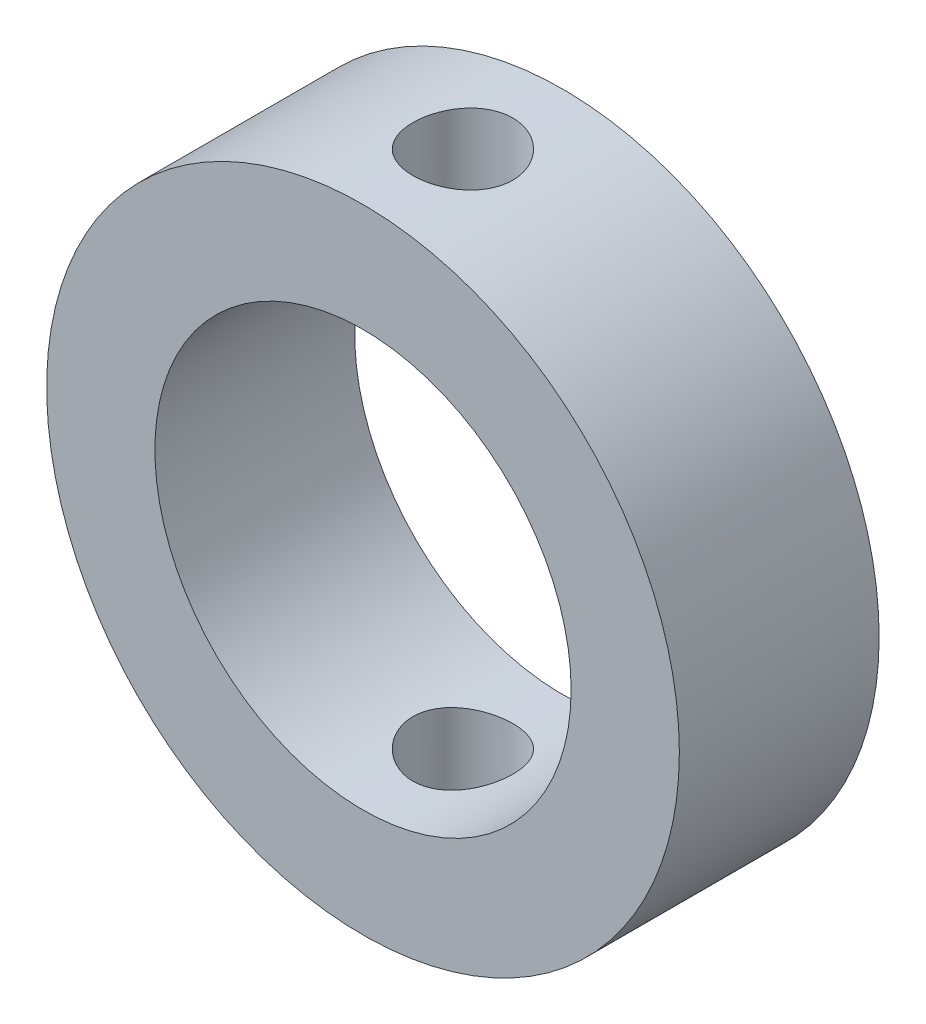
from build123d import *

# Parameters (mm, degrees)
COLLAR_RING_SKETCH_R     = 19
COLLAR_RING_SKETCH_R_2   = 12.5
COLLAR_RING_38X_25_DEPTH = 12
CROSS_HOLE_6_DEPTH       = 30.427877939
CROSS_HOLE_6_DEPTH_BACK  = 30.427877939
CROSS_HOLE_SKETCH_R      = 3


with BuildPart() as part:
    # Collar Ring Sketch → Collar Ring Ø38xØ25 (new body)
    with BuildSketch(Plane.XY):
        Circle(COLLAR_RING_SKETCH_R)
        Circle(COLLAR_RING_SKETCH_R_2, mode=Mode.SUBTRACT)
    extrude(amount=COLLAR_RING_38X_25_DEPTH)

    # Cross Hole Sketch → Cross Hole Ø6 (cut, two sides: drawn at the far end of the back side and taken through both)
    with BuildSketch(Plane(origin=(0, 0, 0), x_dir=(1, 0, 0), z_dir=(0, 1, 0)).offset(-CROSS_HOLE_6_DEPTH_BACK)):
        with Locations(Location((0, -6, 0), (0, 0, 270))):
            Circle(CROSS_HOLE_SKETCH_R)
    extrude(amount=CROSS_HOLE_6_DEPTH + CROSS_HOLE_6_DEPTH_BACK, mode=Mode.SUBTRACT)


solid = part.part
